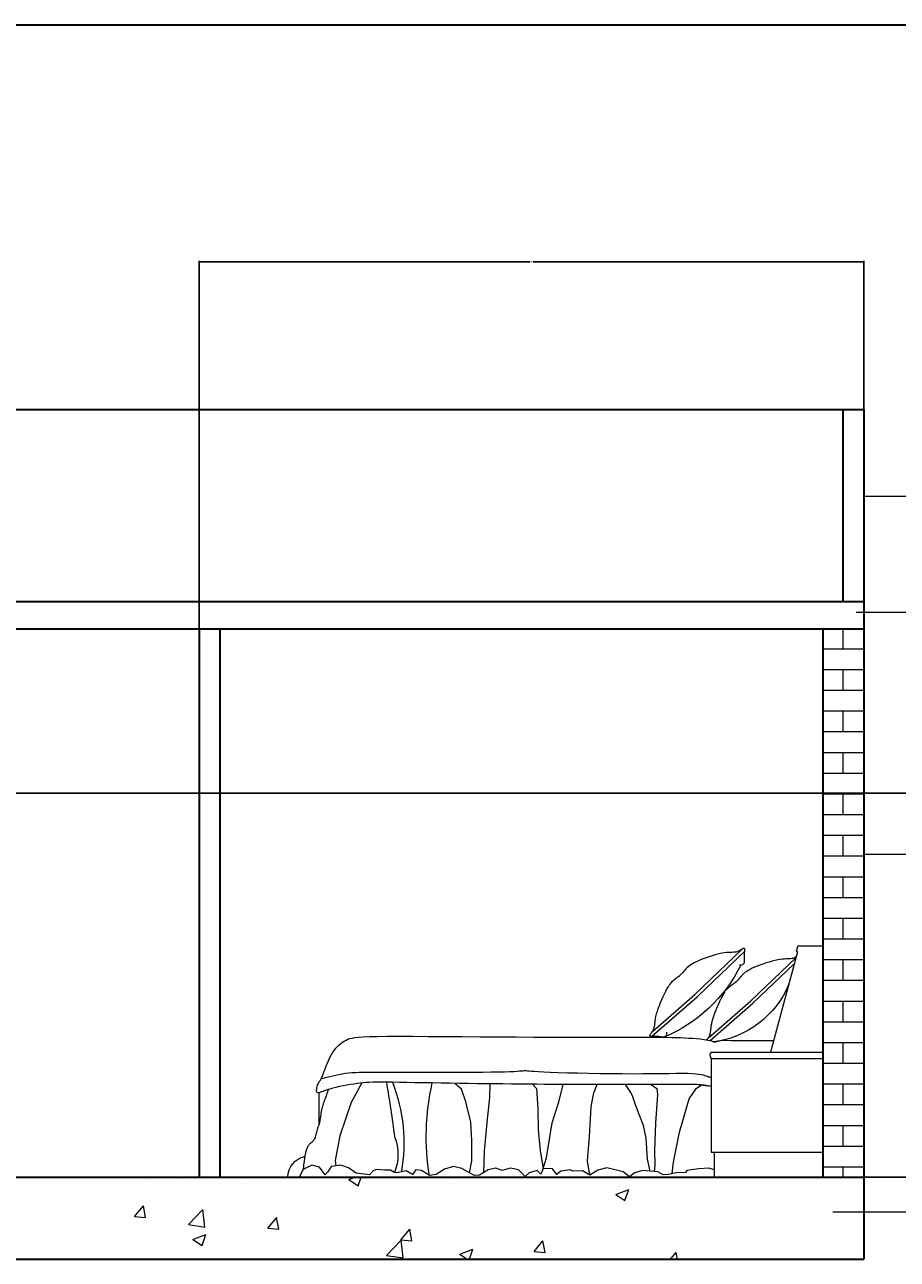
# Model space of a CAD drawing. Units: inches. Extents: x 2250 to 3547, y 1387 to 2604.
# Tile 10 of 11: x 3100 to 3291, y 2334 to 2604. Entities that reach past the tile are written whole.
import ezdxf

# ---------------------------------------------------------------- set-up
doc = ezdxf.new("R2010")
doc.units = ezdxf.units.IN
for name, color, linetype, lineweight in [('A-ANNO-DIMS', 2, 'Continuous', 18), ('A-ANNO-TEXT', 7, 'Continuous', 18), ('A-ANNO-TTLB', 7, 'Continuous', 35), ('A-FLOR-PATT', 252, 'Continuous', 13), ('A-FURN', 9, 'Continuous', 18), ('A-SECT', 7, 'Continuous', 35), ('A-WALL-PATT', 252, 'Continuous', 13)]:
    doc.layers.add(name, color=color, linetype=linetype, lineweight=lineweight)
doc.styles.get("Standard").update_dxf_attribs({"font": 'arial.ttf'})
doc.dimstyles.get("Standard").update_dxf_attribs({"dimtxt": 0.18, "dimasz": 0.18, "dimexe": 0.18, "dimexo": 0.0625, "dimgap": 0.09, "dimtad": 0, "dimtih": 1, "dimtoh": 1, "dimdec": 4, "dimzin": 0, "dimdsep": 46, "dimtxsty": 'Standard', "dimcen": 0.09, "dimadec": 0, "dimazin": 0, "dimtfac": 1, "dimtdec": 4, "dimtofl": 0, "dimtmove": 0, "dimatfit": 3, "dimfxl": 1, "dimtolj": 1, "dimtzin": 0, "dimarcsym": 0})

# ---------------------------------------------------------------- blocks, each defined once
blk = doc.blocks.new('A$C08BC4B9A')
for p, q in [((0, 924.5), (0.5, 925)), ((0, 0), (0, 924.5)), ((95, 925), (0.5, 925)), ((101.1, 921.9), (105, 907.4)), ((101.4, 901.2), (208.9, 500)), ((311.4, 909.3), (311.5, 910.8)), ((311.5, 907.6), (311.4, 909.3)), ((311.5, 910.8), (311.7, 912.1)), ((311.7, 905.6), (311.5, 907.6)), ((311.7, 912.1), (312.1, 913.2)), ((312, 903.5), (311.7, 905.6)), ((502.9, 721.7), (311.9, 904.5)), ((312.3, 901.1), (312, 903.5)), ((312.1, 913.2), (312.7, 914.1)), ((312.6, 898.6), (312.3, 901.1)), ((312.9, 895.9), (312.6, 898.6)), ((312.7, 914.1), (313.6, 914.7)), ((313.1, 892.9), (312.9, 895.9)), ((313.3, 889.8), (313.1, 892.9)), ((313.4, 886.5), (313.3, 889.8)), ((313.6, 914.7), (314.7, 915)), ((314.7, 915), (316, 915.1)), ((316, 915.1), (317.6, 914.9)), ((317.6, 914.9), (319.3, 914.5)), ((319.3, 914.5), (321.1, 913.7)), ((511.6, 731.1), (320.5, 913.9)), ((321.1, 913.7), (323.2, 912.6)), ((323.2, 912.6), (325.4, 911.2)), ((325.4, 911.2), (327.8, 909.6)), ((327.8, 909.6), (330.4, 907.8)), ((330.4, 907.8), (333.3, 906.1)), ((333.3, 906.1), (336.4, 904.3)), ((336.4, 904.3), (339.9, 902.7)), ((339.9, 902.7), (343.7, 901.4)), ((343.7, 901.4), (347.9, 900.4)), ((347.9, 900.4), (352.5, 899.8)), ((352.5, 899.8), (357.6, 899.5)), ((357.6, 899.5), (363.2, 899.4)), ((363.2, 899.4), (369.6, 899.2)), ((369.6, 899.2), (376.7, 898.9)), ((376.7, 898.9), (384.6, 898.3)), ((384.6, 898.3), (393.4, 897.3)), ((393.4, 897.3), (403.3, 895.7)), ((403.3, 895.7), (414.2, 893.3)), ((414.2, 893.3), (425.9, 890.4)), ((425.9, 890.4), (438.1, 886.9)), ((106.6, 881.7), (106.8, 881.6)), ((106.8, 881.6), (109.7, 879.8)), ((288, 704.9), (107.8, 877.3)), ((109.7, 879.8), (112.8, 878.1)), ((112.8, 878.1), (116.3, 876.5)), ((279.2, 695.5), (114.2, 853.4)), ((116.3, 876.5), (120.1, 875.2)), ((120.1, 875.2), (124.3, 874.2)), ((124.3, 874.2), (128.9, 873.6)), ((128.9, 873.6), (134, 873.3)), ((134, 873.3), (139.6, 873.2)), ((139.6, 873.2), (146, 873)), ((146, 873), (153.1, 872.7)), ((153.1, 872.7), (161, 872.1)), ((161, 872.1), (169.8, 871.1)), ((169.8, 871.1), (179.7, 869.5)), ((179.7, 869.5), (190.6, 867.1)), ((190.6, 867.1), (202.3, 864.2)), ((202.3, 864.2), (214.5, 860.7)), ((214.5, 860.7), (226.9, 856.8)), ((226.9, 856.8), (239.3, 852.7)), ((239.3, 852.7), (251.3, 848.4)), ((251.3, 848.4), (262.7, 844)), ((262.7, 844), (273.2, 839.6)), ((312.7, 863.2), (312.8, 867.3)), ((313.1, 859.2), (312.7, 863.2)), ((312.8, 867.3), (313, 871.5)), ((313, 871.5), (313.3, 875.5)), ((314.3, 855.7), (313.1, 859.2)), ((313.3, 875.5), (313.4, 879.4)), ((313.4, 883), (313.4, 886.5)), ((313.4, 879.4), (313.4, 883)), ((316.7, 852.8), (314.3, 855.7)), ((320.4, 850.8), (316.7, 852.8)), ((325.8, 849.7), (320.4, 850.8)), ((333.2, 849.9), (325.8, 849.7)), ((438.1, 886.9), (450.5, 883.1)), ((450.5, 883.1), (462.9, 878.9)), ((462.9, 878.9), (474.9, 874.6)), ((474.9, 874.6), (486.3, 870.2)), ((486.3, 870.2), (496.8, 865.9)), ((496.8, 865.9), (506.1, 861.7)), ((506.1, 861.7), (514.3, 857.6)), ((514.3, 857.6), (521.6, 853.6)), ((521.6, 853.6), (528, 849.7)), ((528, 849.7), (533.7, 845.7)), ((533.7, 845.7), (538.8, 841.7)), ((538.8, 841.7), (543.4, 837.5)), ((273.2, 839.6), (282.5, 835.5)), ((282.5, 835.5), (290.7, 831.4)), ((290.7, 831.4), (298, 827.4)), ((298, 827.4), (304.4, 823.4)), ((304.4, 823.4), (310.1, 819.5)), ((310.1, 819.5), (315.2, 815.4)), ((315.2, 815.4), (319.8, 811.3)), ((319.8, 811.3), (324.1, 807)), ((324.1, 807), (328.1, 802.5)), ((328.1, 802.5), (332, 797.9)), ((332, 797.9), (335.8, 793.2)), ((335.8, 793.2), (339.7, 788.4)), ((543.4, 837.5), (547.7, 833.2)), ((547.7, 833.2), (551.7, 828.7)), ((551.7, 828.7), (555.6, 824.1)), ((555.6, 824.1), (559.4, 819.4)), ((559.4, 819.4), (563.3, 814.6)), ((563.3, 814.6), (567.7, 810.4)), ((572.2, 806.3), (567.7, 810.4)), ((577.3, 802.8), (572.2, 806.3)), ((582.3, 799.4), (577.3, 802.8)), ((587.2, 795.8), (582.3, 799.4)), ((592, 792.2), (587.2, 795.8)), ((596.6, 788.2), (592, 792.2)), ((339.7, 788.4), (344.1, 784.1)), ((344.2, 784), (344.1, 784.1)), ((344.5, 783.8), (344.2, 784)), ((344.9, 783.4), (344.5, 783.8)), ((345.5, 782.9), (344.9, 783.4)), ((346.1, 782.3), (345.5, 782.9)), ((346.8, 781.7), (346.1, 782.3)), ((347.6, 781.1), (346.8, 781.7)), ((348.3, 780.5), (347.6, 781.1)), ((349.1, 779.9), (348.3, 780.5)), ((349.8, 779.4), (349.1, 779.9)), ((350.5, 778.9), (349.8, 779.4)), ((351.1, 778.4), (350.5, 778.9)), ((351.8, 777.9), (351.1, 778.4)), ((352.4, 777.5), (351.8, 777.9)), ((353.1, 777), (352.4, 777.5)), ((353.7, 776.6), (353.1, 777)), ((354.3, 776.2), (353.7, 776.6)), ((354.9, 775.7), (354.3, 776.2)), ((355.6, 775.3), (354.9, 775.7)), ((356.2, 774.9), (355.6, 775.3)), ((356.8, 774.4), (356.2, 774.9)), ((357.4, 774), (356.8, 774.4)), ((358.1, 773.6), (357.4, 774)), ((358.7, 773.1), (358.1, 773.6)), ((359.3, 772.7), (358.7, 773.1)), ((359.9, 772.3), (359.3, 772.7)), ((360.5, 771.8), (359.9, 772.3)), ((361.2, 771.4), (360.5, 771.8)), ((361.8, 770.9), (361.2, 771.4)), ((362.4, 770.5), (361.8, 770.9)), ((363, 770), (362.4, 770.5)), ((363.6, 769.6), (363, 770)), ((364.2, 769.1), (363.6, 769.6)), ((364.8, 768.7), (364.2, 769.1)), ((365.4, 768.2), (364.8, 768.7)), ((366, 767.8), (365.4, 768.2)), ((366.6, 767.3), (366, 767.8)), ((367.2, 766.8), (366.6, 767.3)), ((367.8, 766.4), (367.2, 766.8)), ((368.3, 765.9), (367.8, 766.4)), ((368.9, 765.4), (368.3, 765.9)), ((369.5, 764.9), (368.9, 765.4)), ((370.1, 764.4), (369.5, 764.9)), ((370.7, 763.9), (370.1, 764.4)), ((371.2, 763.5), (370.7, 763.9)), ((371.8, 763), (371.2, 763.5)), ((372.4, 762.4), (371.8, 763)), ((373, 761.9), (372.4, 762.4)), ((373.5, 761.4), (373, 761.9)), ((374.1, 760.9), (373.5, 761.4)), ((374.7, 760.4), (374.1, 760.9)), ((375.2, 759.8), (374.7, 760.4)), ((375.8, 759.3), (375.2, 759.8)), ((376.3, 758.7), (375.8, 759.3)), ((376.9, 758.2), (376.3, 758.7)), ((377.4, 757.6), (376.9, 758.2)), ((378, 757), (377.4, 757.6)), ((378.6, 756.5), (378, 757)), ((379.2, 755.8), (378.6, 756.5)), ((379.8, 755.2), (379.2, 755.8)), ((380.5, 754.5), (379.8, 755.2)), ((381.3, 753.8), (380.5, 754.5)), ((382.2, 753.1), (381.3, 753.8)), ((383.2, 752.3), (382.2, 753.1)), ((384.2, 751.4), (383.2, 752.3)), ((385.4, 750.5), (384.2, 751.4)), ((386.6, 749.6), (385.4, 750.5)), ((387.8, 748.7), (386.6, 749.6)), ((388.9, 747.8), (387.8, 748.7)), ((389.9, 746.9), (388.9, 747.8)), ((390.8, 746), (389.9, 746.9)), ((391.4, 745.3), (390.8, 746)), ((391.9, 744.6), (391.4, 745.3)), ((392.1, 744), (391.9, 744.6)), ((392, 741.9), (392.1, 742.4)), ((392, 741.3), (392, 741.9)), ((392, 740.8), (392, 741.3)), ((392.2, 743.4), (392.1, 744)), ((392.1, 742.4), (392.2, 742.9)), ((392.2, 742.9), (392.2, 743.4)), ((601.1, 783.9), (596.6, 788.2)), ((605.5, 779.1), (601.1, 783.9)), ((609.9, 773.7), (605.5, 779.1)), ((614.3, 767.6), (609.9, 773.7)), ((618.8, 760.7), (614.3, 767.6)), ((623.5, 752.8), (618.8, 760.7)), ((628.4, 743.8), (623.5, 752.8)), ((633.5, 733.7), (628.4, 743.8)), ((450.1, 546.6), (279.2, 695.5)), ((457.7, 557), (288, 704.9)), ((392.1, 740.1), (392, 740.8)), ((392.4, 739.4), (392.1, 740.1)), ((392.7, 738.6), (392.4, 739.4)), ((393.1, 737.8), (392.7, 738.6)), ((393.6, 737), (393.1, 737.8)), ((394.1, 736.1), (393.6, 737)), ((394.7, 735.2), (394.1, 736.1)), ((395.2, 734.3), (394.7, 735.2)), ((395.8, 733.4), (395.2, 734.3)), ((396.4, 732.4), (395.8, 733.4)), ((397, 731.5), (396.4, 732.4)), ((397.6, 730.5), (397, 731.5)), ((398.2, 729.5), (397.6, 730.5)), ((398.7, 728.5), (398.2, 729.5)), ((399.3, 727.4), (398.7, 728.5)), ((399.9, 726.4), (399.3, 727.4)), ((400.5, 725.3), (399.9, 726.4)), ((401.1, 724.3), (400.5, 725.3)), ((401.7, 723.2), (401.1, 724.3)), ((402.4, 722), (401.7, 723.2)), ((403, 720.9), (402.4, 722)), ((403.6, 719.8), (403, 720.9)), ((404.2, 718.6), (403.6, 719.8)), ((404.8, 717.4), (404.2, 718.6)), ((405.4, 716.2), (404.8, 717.4)), ((406.1, 715), (405.4, 716.2)), ((406.7, 713.8), (406.1, 715)), ((407.3, 712.5), (406.7, 713.8)), ((408, 711.2), (407.3, 712.5)), ((408.6, 710), (408, 711.2)), ((409.3, 708.7), (408.6, 710)), ((409.9, 707.3), (409.3, 708.7)), ((410.6, 706), (409.9, 707.3)), ((411.2, 704.7), (410.6, 706)), ((411.9, 703.3), (411.2, 704.7)), ((412.5, 701.9), (411.9, 703.3)), ((413.2, 700.6), (412.5, 701.9)), ((413.8, 699.2), (413.2, 700.6)), ((414.5, 697.8), (413.8, 699.2)), ((415.1, 696.4), (414.5, 697.8)), ((415.8, 694.9), (415.1, 696.4)), ((416.4, 693.5), (415.8, 694.9)), ((417.1, 692.1), (416.4, 693.5)), ((417.7, 690.6), (417.1, 692.1)), ((685.7, 562.3), (502.9, 721.7)), ((681.3, 583.2), (511.6, 731.1)), ((638.7, 722.7), (633.5, 733.7)), ((643.9, 711), (638.7, 722.7)), ((649, 699), (643.9, 711)), ((653.8, 686.9), (649, 699)), ((418.4, 689.2), (417.7, 690.6)), ((419, 687.7), (418.4, 689.2)), ((419.7, 686.2), (419, 687.7)), ((420.3, 684.7), (419.7, 686.2)), ((421, 683.3), (420.3, 684.7)), ((421.6, 681.8), (421, 683.3)), ((422.2, 680.3), (421.6, 681.8)), ((422.9, 678.8), (422.2, 680.3)), ((423.5, 677.3), (422.9, 678.8)), ((424.1, 675.8), (423.5, 677.3)), ((424.7, 674.3), (424.1, 675.8)), ((425.4, 672.8), (424.7, 674.3)), ((426, 671.3), (425.4, 672.8)), ((426.6, 669.7), (426, 671.3)), ((427.2, 668.2), (426.6, 669.7)), ((427.8, 666.7), (427.2, 668.2)), ((428.4, 665.2), (427.8, 666.7)), ((429, 663.7), (428.4, 665.2)), ((429.6, 662.2), (429, 663.7)), ((430.1, 660.7), (429.6, 662.2)), ((430.7, 659.2), (430.1, 660.7)), ((431.3, 657.7), (430.7, 659.2)), ((431.8, 656.2), (431.3, 657.7)), ((432.4, 654.7), (431.8, 656.2)), ((432.9, 653.2), (432.4, 654.7)), ((433.4, 651.8), (432.9, 653.2)), ((434, 650.3), (433.4, 651.8)), ((434.5, 648.8), (434, 650.3)), ((435, 647.4), (434.5, 648.8)), ((435.5, 645.9), (435, 647.4)), ((436, 644.5), (435.5, 645.9)), ((436.5, 643.1), (436, 644.5)), ((436.9, 641.7), (436.5, 643.1)), ((658.2, 675), (653.8, 686.9)), ((662, 663.6), (658.2, 675)), ((665.2, 652.9), (662, 663.6)), ((667.5, 643.2), (665.2, 652.9)), ((669.2, 634.4), (667.5, 643.2)), ((437.4, 640.2), (436.9, 641.7)), ((437.9, 638.8), (437.4, 640.2)), ((438.3, 637.5), (437.9, 638.8)), ((438.7, 636.1), (438.3, 637.5)), ((439.1, 634.7), (438.7, 636.1)), ((439.6, 633.4), (439.1, 634.7)), ((440, 632), (439.6, 633.4)), ((440.3, 630.7), (440, 632)), ((440.7, 629.4), (440.3, 630.7)), ((441.1, 628.1), (440.7, 629.4)), ((441.4, 626.8), (441.1, 628.1)), ((441.8, 625.5), (441.4, 626.8)), ((442.1, 624.3), (441.8, 625.5)), ((442.4, 623.1), (442.1, 624.3)), ((442.7, 621.8), (442.4, 623.1)), ((443, 620.6), (442.7, 621.8)), ((443.3, 619.4), (443, 620.6)), ((443.6, 618.3), (443.3, 619.4)), ((443.8, 617.1), (443.6, 618.3)), ((444.1, 616), (443.8, 617.1)), ((444.3, 614.8), (444.1, 616)), ((444.5, 613.7), (444.3, 614.8)), ((444.7, 612.6), (444.5, 613.7)), ((445, 611.5), (444.7, 612.6)), ((445.2, 610.5), (445, 611.5)), ((445.4, 609.4), (445.2, 610.5)), ((445.5, 608.4), (445.4, 609.4)), ((445.7, 607.3), (445.5, 608.4)), ((445.9, 606.3), (445.7, 607.3)), ((446, 605.3), (445.9, 606.3)), ((446.2, 604.3), (446, 605.3)), ((446.4, 603.3), (446.2, 604.3)), ((446.5, 602.4), (446.4, 603.3)), ((446.6, 601.4), (446.5, 602.4)), ((446.8, 600.5), (446.6, 601.4)), ((446.9, 599.6), (446.8, 600.5)), ((447, 598.6), (446.9, 599.6)), ((447.1, 597.7), (447, 598.6)), ((447.2, 596.9), (447.1, 597.7)), ((447.3, 596), (447.2, 596.9)), ((447.4, 595.1), (447.3, 596)), ((447.5, 594.3), (447.4, 595.1)), ((447.6, 593.4), (447.5, 594.3)), ((447.7, 592.6), (447.6, 593.4)), ((670.4, 626.6), (669.2, 634.4)), ((671.3, 619.5), (670.4, 626.6)), ((671.9, 613.2), (671.3, 619.5)), ((672.5, 607.6), (671.9, 613.2)), ((673.1, 602.5), (672.5, 607.6)), ((674.1, 598), (673.1, 602.5)), ((675.4, 593.9), (674.1, 598)), ((677, 590.2), (675.4, 593.9)), ((366.1, 546.8), (196.6, 546.1)), ((400.7, 547.5), (366.1, 546.8)), ((420, 543.6), (400.7, 547.5)), ((431.7, 540.1), (420, 543.6)), ((445.4, 545.7), (439.4, 542.5)), ((460.2, 548.4), (445.4, 545.7)), ((447.8, 591.8), (447.7, 592.6)), ((447.9, 591), (447.8, 591.8)), ((448, 590.2), (447.9, 591)), ((448, 589.4), (448, 590.2)), ((448.1, 588.6), (448, 589.4)), ((448.2, 587.9), (448.1, 588.6)), ((448.3, 587.1), (448.2, 587.9)), ((448.3, 586.4), (448.3, 587.1)), ((448.4, 585.6), (448.3, 586.4)), ((448.5, 584.9), (448.4, 585.6)), ((448.6, 584.2), (448.5, 584.9)), ((448.6, 583.5), (448.6, 584.2)), ((448.7, 582.8), (448.6, 583.5)), ((448.8, 582.1), (448.7, 582.8)), ((448.9, 581.4), (448.8, 582.1)), ((448.9, 580.8), (448.9, 581.4)), ((449, 580.1), (448.9, 580.8)), ((449.1, 579.5), (449, 580.1)), ((449.2, 578.8), (449.1, 579.5)), ((449.3, 578.2), (449.2, 578.8)), ((449.4, 577.6), (449.3, 578.2)), ((449.5, 577), (449.4, 577.6)), ((449.6, 576.4), (449.5, 577)), ((449.7, 575.8), (449.6, 576.4)), ((449.8, 575.2), (449.7, 575.8)), ((449.9, 574.6), (449.8, 575.2)), ((450, 574), (449.9, 574.6)), ((450.1, 573.5), (450, 574)), ((450.3, 572.9), (450.1, 573.5)), ((450.4, 572.4), (450.3, 572.9)), ((450.5, 571.8), (450.4, 572.4)), ((450.7, 571.3), (450.5, 571.8)), ((450.8, 570.8), (450.7, 571.3)), ((451, 570.2), (450.8, 570.8)), ((451.1, 569.7), (451, 570.2)), ((451.3, 569.2), (451.1, 569.7)), ((451.5, 568.7), (451.3, 569.2)), ((451.6, 568.2), (451.5, 568.7)), ((451.8, 567.7), (451.6, 568.2)), ((452, 567.2), (451.8, 567.7)), ((452.2, 566.8), (452, 567.2)), ((452.4, 566.3), (452.2, 566.8)), ((452.6, 565.8), (452.4, 566.3)), ((452.8, 565.4), (452.6, 565.8)), ((453, 564.9), (452.8, 565.4)), ((453.2, 564.5), (453, 564.9)), ((453.4, 564), (453.2, 564.5)), ((453.6, 563.6), (453.4, 564)), ((453.8, 563.1), (453.6, 563.6)), ((454.1, 562.7), (453.8, 563.1)), ((454.3, 562.3), (454.1, 562.7)), ((454.5, 561.9), (454.3, 562.3)), ((454.8, 561.5), (454.5, 561.9)), ((455, 561.1), (454.8, 561.5)), ((455.2, 560.7), (455, 561.1)), ((455.5, 560.3), (455.2, 560.7)), ((455.7, 559.9), (455.5, 560.3)), ((456, 559.5), (455.7, 559.9)), ((456.2, 559.1), (456, 559.5)), ((456.4, 558.8), (456.2, 559.1)), ((456.7, 558.4), (456.4, 558.8)), ((456.9, 558), (456.7, 558.4)), ((457.2, 557.7), (456.9, 558)), ((457.4, 557.3), (457.2, 557.7)), ((457.7, 557), (457.4, 557.3)), ((457.9, 556.6), (457.7, 557)), ((458.2, 556.3), (457.9, 556.6)), ((458.4, 555.9), (458.2, 556.3)), ((458.7, 555.6), (458.4, 555.9)), ((458.9, 555.3), (458.7, 555.6)), ((459.2, 554.9), (458.9, 555.3)), ((459.4, 554.6), (459.2, 554.9)), ((459.7, 554.3), (459.4, 554.6)), ((459.9, 554), (459.7, 554.3)), ((460.2, 553.6), (459.9, 554)), ((460.4, 553.3), (460.2, 553.6)), ((475.2, 550.7), (460.2, 548.4)), ((460.7, 553), (460.4, 553.3)), ((461, 552.6), (460.7, 553)), ((461.3, 552.3), (461, 552.6)), ((461.6, 551.9), (461.3, 552.3)), ((461.9, 551.5), (461.6, 551.9)), ((462.2, 551.1), (461.9, 551.5)), ((462.5, 550.7), (462.2, 551.1)), ((462.8, 550.3), (462.5, 550.7)), ((463.2, 549.8), (462.8, 550.3)), ((463.5, 549.4), (463.2, 549.8)), ((463.8, 548.9), (463.5, 549.4)), ((490.5, 552.6), (475.2, 550.7)), ((506, 554.2), (490.5, 552.6)), ((521.7, 555.5), (506, 554.2)), ((537.6, 556.6), (521.7, 555.5)), ((553.6, 557.4), (537.6, 556.6)), ((569.7, 558.1), (553.6, 557.4)), ((586, 558.6), (569.7, 558.1)), ((603.2, 559), (586, 558.6)), ((621.8, 559.3), (603.2, 559)), ((642.6, 559.5), (621.8, 559.3)), ((624.8, 579.5), (625.2, 572.1)), ((625.2, 572.1), (626.6, 566.8)), ((626.6, 566.8), (629, 563.3)), ((629, 563.3), (632, 561.2)), ((632, 561.2), (635.6, 560.2)), ((635.6, 560.2), (639.6, 560.1)), ((639.6, 560.1), (643.7, 560.5)), ((666.5, 559.6), (642.6, 559.5)), ((643.7, 560.5), (647.9, 561)), ((647.9, 561), (651.9, 561.6)), ((651.9, 561.6), (655.7, 562)), ((655.7, 562), (659.3, 562.3)), ((659.3, 562.3), (662.8, 562.5)), ((662.8, 562.5), (666.1, 562.7)), ((666.1, 562.7), (669.2, 562.7)), ((693.9, 559.6), (666.5, 559.6)), ((669.2, 562.7), (672.2, 562.7)), ((672.2, 562.7), (674.9, 562.7)), ((674.9, 562.7), (677.5, 562.6)), ((678.8, 586.8), (677, 590.2)), ((677.5, 562.6), (679.8, 562.4)), ((680.8, 583.8), (678.8, 586.8)), ((679.8, 562.4), (682, 562.3)), ((682.8, 581.1), (680.8, 583.8)), ((682, 562.3), (683.9, 562.3)), ((684.7, 578.6), (682.8, 581.1)), ((683.9, 562.3), (685.7, 562.3)), ((686.5, 576.4), (684.7, 578.6)), ((685.7, 562.3), (687.2, 562.4)), ((688.1, 574.3), (686.5, 576.4)), ((687.2, 562.4), (688.5, 562.7)), ((689.3, 572.3), (688.1, 574.3)), ((688.5, 562.7), (689.5, 563.2)), ((690.2, 570.5), (689.3, 572.3)), ((689.5, 563.2), (690.3, 563.9)), ((690.8, 568.8), (690.2, 570.5)), ((690.3, 563.9), (690.9, 564.9)), ((691.1, 567.3), (690.8, 568.8)), ((690.9, 564.9), (691.1, 566)), ((691.1, 566), (691.1, 567.3)), ((725.8, 559.7), (693.9, 559.6)), ((762.8, 559.7), (725.8, 559.7)), ((805.4, 559.7), (762.8, 559.7)), ((853.4, 559.7), (805.4, 559.7)), ((906.2, 559.7), (853.4, 559.7)), ((963.4, 559.8), (906.2, 559.7)), ((1024.6, 559.9), (963.4, 559.8)), ((1089.2, 560.1), (1024.6, 559.9)), ((1156.7, 560.4), (1089.2, 560.1)), ((1226.8, 560.7), (1156.7, 560.4)), ((1298.7, 561.1), (1226.8, 560.7)), ((1371.2, 561.6), (1298.7, 561.1)), ((1443.1, 562.1), (1371.2, 561.6)), ((1512.8, 562.6), (1443.1, 562.1)), ((1579.1, 563), (1512.8, 562.6)), ((1640.5, 563.3), (1579.1, 563)), ((1695.8, 563.4), (1640.5, 563.3)), ((1743.5, 563.3), (1695.8, 563.4)), ((1782.8, 563), (1743.5, 563.3)), ((1814.2, 562.4), (1782.8, 563)), ((1838.9, 561.5), (1814.2, 562.4)), ((1858, 560.2), (1838.9, 561.5)), ((1872.6, 558.6), (1858, 560.2)), ((1883.7, 556.6), (1872.6, 558.6)), ((1892.6, 554.2), (1883.7, 556.6)), ((1900.3, 551.3), (1892.6, 554.2)), ((1907.7, 547.9), (1900.3, 551.3)), ((1915, 544), (1907.7, 547.9)), ((1922.1, 539.6), (1915, 544)), ((445.9, 500), (0, 500)), ((439.4, 542.5), (431.7, 540.1)), ((1929, 534.5), (1922.1, 539.6)), ((1935.8, 528.9), (1929, 534.5)), ((1942.3, 522.6), (1935.8, 528.9)), ((1948.6, 515.6), (1942.3, 522.6)), ((1954.6, 508), (1948.6, 515.6)), ((1960.4, 499.6), (1954.6, 508)), ((1965.8, 490.7), (1960.4, 499.6)), ((445.9, 475), (0, 475)), ((445.9, 475), (445.9, 100)), ((1970.9, 481.5), (1965.8, 490.7)), ((1975.6, 472.1), (1970.9, 481.5)), ((1980, 462.7), (1975.6, 472.1)), ((1984, 453.6), (1980, 462.7)), ((1987.5, 445), (1984, 453.6)), ((1990.7, 437), (1987.5, 445)), ((445.9, 397.8), (449.1, 398.3)), ((449.1, 398.3), (453.4, 399.2)), ((453.4, 399.2), (457.6, 400.4)), ((457.6, 400.4), (461.8, 402)), ((461.8, 402), (466.2, 403.7)), ((466.2, 403.7), (471.3, 405.6)), ((471.3, 405.6), (477.6, 407.5)), ((477.6, 407.5), (485.4, 409.4)), ((485.4, 409.4), (495.3, 411.1)), ((495.3, 411.1), (507.7, 412.5)), ((507.7, 412.5), (523, 413.5)), ((523, 413.5), (541.5, 414)), ((541.5, 414), (563.2, 414.2)), ((563.2, 414.2), (588.2, 414.1)), ((588.2, 414.1), (616.4, 413.7)), ((616.4, 413.7), (647.7, 413.3)), ((647.7, 413.3), (682, 412.9)), ((682, 412.9), (719.4, 412.6)), ((719.4, 412.6), (759.7, 412.4)), ((759.7, 412.4), (802.6, 412.6)), ((802.6, 412.6), (847.4, 413)), ((847.4, 413), (892.8, 413.6)), ((892.8, 413.6), (937.8, 414.4)), ((937.8, 414.4), (981.1, 415.3)), ((981.1, 415.3), (1021.7, 416.4)), ((1021.7, 416.4), (1058.6, 417.5)), ((1058.6, 417.5), (1090.4, 418.7)), ((1090.4, 418.7), (1116.5, 419.9)), ((1116.5, 419.9), (1137.2, 421)), ((1137.2, 421), (1153.4, 422.1)), ((1153.4, 422.1), (1165.7, 423)), ((1165.7, 423), (1174.9, 423.8)), ((1174.9, 423.8), (1181.7, 424.4)), ((1181.7, 424.4), (1186.9, 424.8)), ((1186.9, 424.8), (1191.2, 425)), ((1191.2, 425), (1195.4, 424.8)), ((1195.4, 424.8), (1200, 424.5)), ((1200, 424.5), (1205.8, 423.9)), ((1205.8, 423.9), (1213.3, 423.2)), ((1213.3, 423.2), (1223.1, 422.4)), ((1223.1, 422.4), (1236, 421.7)), ((1236, 421.7), (1252.5, 420.9)), ((1252.5, 420.9), (1273.3, 420.3)), ((1273.3, 420.3), (1298.7, 419.7)), ((1298.7, 419.7), (1328.3, 419.4)), ((1328.3, 419.4), (1361.1, 419.1)), ((1361.1, 419.1), (1396.4, 418.9)), ((1396.4, 418.9), (1433.4, 418.8)), ((1433.4, 418.8), (1471.3, 418.7)), ((1471.3, 418.7), (1509.3, 418.7)), ((1509.3, 418.7), (1546.6, 418.7)), ((1546.6, 418.7), (1582.4, 418.7)), ((1582.4, 418.7), (1616.7, 418.7)), ((1616.7, 418.7), (1649.3, 418.7)), ((1649.3, 418.7), (1680.1, 418.7)), ((1680.1, 418.7), (1709, 418.7)), ((1709, 418.7), (1736, 418.7)), ((1736, 418.7), (1760.9, 418.7)), ((1760.9, 418.7), (1783.8, 418.7)), ((1783.8, 418.7), (1804.5, 418.7)), ((1804.5, 418.7), (1823.2, 418.6)), ((1823.2, 418.6), (1840.3, 418.5)), ((1840.3, 418.5), (1856.1, 418.1)), ((1856.1, 418.1), (1870.7, 417.6)), ((1870.7, 417.6), (1884.5, 416.7)), ((1884.5, 416.7), (1897.8, 415.6)), ((1897.8, 415.6), (1910.8, 414)), ((1910.8, 414), (1923.7, 412)), ((1923.7, 412), (1936.5, 409.7)), ((1936.5, 409.7), (1949.1, 407.1)), ((1949.1, 407.1), (1961.3, 404.4)), ((1961.3, 404.4), (1973.1, 401.6)), ((1973.1, 401.6), (1984.4, 398.8)), ((1984.4, 398.8), (1995, 396.1)), ((1993.4, 429.7), (1990.7, 437)), ((1995.8, 423.3), (1993.4, 429.7)), ((1995, 396.1), (2004.8, 393.6)), ((1997.8, 417.5), (1995.8, 423.3)), ((1999.6, 412.4), (1997.8, 417.5)), ((2001.3, 407.8), (1999.6, 412.4)), ((2002.8, 403.7), (2001.3, 407.8)), ((2004.3, 400.1), (2002.8, 403.7)), ((2005.8, 396.8), (2004.3, 400.1)), ((2007.5, 393.8), (2005.8, 396.8)), ((445.9, 362), (481.5, 369.7)), ((445.9, 362.5), (450.4, 363.2)), ((450.4, 363.2), (457.2, 364.1)), ((457.2, 364.1), (463.4, 364.9)), ((463.4, 364.9), (468.9, 365.7)), ((468.9, 365.7), (473.6, 366.4)), ((473.6, 366.4), (477.6, 367.1)), ((477.6, 367.1), (481.1, 367.7)), ((481.1, 367.7), (484.4, 368.3)), ((484.4, 368.3), (488, 368.8)), ((504.7, 356.4), (486.2, 368.5)), ((488, 368.8), (492.3, 369.2)), ((492.3, 369.2), (497.5, 369.6)), ((497.5, 369.6), (504.1, 369.9)), ((504.1, 369.9), (512.5, 370.1)), ((534.3, 312.8), (504.7, 356.4)), ((512.5, 370.1), (522.9, 370.3)), ((522.9, 370.3), (535.3, 370.3)), ((535.3, 370.3), (549.5, 370.3)), ((549.5, 370.3), (565.4, 370.3)), ((565.4, 370.3), (582.8, 370.2)), ((582.8, 370.2), (601.6, 370.2)), ((601.6, 370.2), (621.6, 370.1)), ((621.6, 370.1), (642.7, 370.1)), ((642.7, 370.1), (664.7, 370.1)), ((663.6, 354.7), (661.8, 330.2)), ((687.3, 370.2), (663.6, 354.7)), ((664.7, 370.1), (687.3, 370.2)), ((687.3, 370.2), (710.4, 370.3)), ((710.4, 370.3), (733.4, 370.4)), ((733.4, 370.4), (756.3, 370.4)), ((756.3, 370.4), (778.7, 370.5)), ((768.3, 339), (789.4, 370.5)), ((778.7, 370.5), (800.2, 370.6)), ((800.2, 370.6), (820.7, 370.6)), ((820.7, 370.6), (840, 370.6)), ((840, 370.6), (858.3, 370.5)), ((858.3, 370.5), (876.2, 370.4)), ((876.2, 370.4), (894, 370.4)), ((894, 370.4), (912.3, 370.3)), ((916.7, 337.2), (903.2, 370.3)), ((912.3, 370.3), (931.5, 370.2)), ((931.5, 370.2), (952, 370.2)), ((952, 370.2), (974.3, 370.2)), ((974.3, 370.2), (998.7, 370.3)), ((998.7, 370.3), (1025.1, 370.4)), ((1025.1, 370.4), (1053.2, 370.6)), ((1054.7, 305.8), (1039.1, 370.5)), ((1053.2, 370.6), (1082.9, 370.8)), ((1082.9, 370.8), (1113.8, 371)), ((1113.8, 371), (1145.8, 371.3)), ((1145.5, 354.7), (1140.2, 274.4)), ((1162.2, 371.4), (1145.5, 354.7)), ((1145.8, 371.3), (1178.6, 371.6)), ((1178.6, 371.6), (1212, 371.9)), ((1212, 371.9), (1245.7, 372.2)), ((1245.7, 372.2), (1279.8, 372.6)), ((1279.8, 372.6), (1314.1, 373)), ((1314.1, 373), (1348.8, 373.4)), ((1332.3, 318), (1331.5, 373.2)), ((1348.8, 373.4), (1383.8, 373.8)), ((1383.8, 373.8), (1419.1, 374.3)), ((1419.1, 374.3), (1454.7, 374.8)), ((1428.3, 300.6), (1445.8, 351.2)), ((1445.8, 351.2), (1472.7, 375.1)), ((1454.7, 374.8), (1490.6, 375.4)), ((1490.6, 375.4), (1526.8, 376)), ((1526.8, 376), (1562.7, 376.6)), ((1562.7, 376.6), (1597.9, 377.2)), ((1597.9, 377.2), (1632, 377.8)), ((1632, 377.8), (1664.4, 378.4)), ((1664.4, 378.4), (1694.6, 378.9)), ((1694.6, 378.9), (1722.2, 379.3)), ((1722.2, 379.3), (1746.7, 379.5)), ((1746.7, 379.5), (1767.7, 379.7)), ((1767.7, 379.7), (1785.7, 379.6)), ((1785.7, 379.6), (1801.2, 379.4)), ((1801.2, 379.4), (1814.9, 378.9)), ((1814.9, 378.9), (1827.4, 378.2)), ((1827.4, 378.2), (1839.2, 377.2)), ((1839.2, 377.2), (1850.9, 375.9)), ((1845.1, 376.6), (1887, 298.9)), ((1850.9, 375.9), (1863.2, 374.3)), ((1863.2, 374.3), (1876.4, 372.4)), ((1876.4, 372.4), (1890.5, 370.2)), ((1890.5, 370.2), (1905, 367.7)), ((1905, 367.7), (1919.7, 364.9)), ((1919.7, 364.9), (1934.2, 362)), ((1934.2, 362), (1948.2, 358.9)), ((1948.2, 358.9), (1961.4, 355.7)), ((1961.4, 355.7), (1973.5, 352.4)), ((1973.5, 352.4), (1984.1, 349.1)), ((1977.1, 352.6), (1976.8, 353.5)), ((1978, 350), (1977.1, 352.6)), ((1979.4, 346.1), (1978, 350)), ((1981.2, 341.1), (1979.4, 346.1)), ((1984.1, 349.1), (1993.3, 345.9)), ((2009.2, 390.9), (2007.5, 393.8)), ((2010.9, 388.2), (2009.2, 390.9)), ((2012.7, 385.4), (2010.9, 388.2)), ((2014.5, 382.5), (2012.7, 385.4)), ((2016.4, 379.3), (2014.5, 382.5)), ((2018.2, 375.7), (2016.4, 379.3)), ((2020, 371.7), (2018.2, 375.7)), ((2021.7, 367.2), (2020, 371.7)), ((2023.2, 362.2), (2021.7, 367.2)), ((2024.6, 357.2), (2023.2, 362.2)), ((2025.5, 352.3), (2024.6, 357.2)), ((2026, 347.7), (2025.5, 352.3)), ((2025.9, 343.7), (2026, 347.7)), ((551.8, 253.5), (534.3, 312.8)), ((661.8, 330.2), (668.8, 215.1)), ((750.9, 293.6), (759.6, 321.5)), ((759.6, 321.5), (768.3, 339)), ((927.2, 283.1), (916.7, 337.2)), ((1082.6, 216.8), (1054.7, 305.8)), ((1342.8, 218.6), (1332.3, 318)), ((1409.1, 220.3), (1428.3, 300.6)), ((1887, 298.9), (1932.4, 164.5)), ((1983.2, 335.3), (1981.2, 341.1)), ((1985.5, 329), (1983.2, 335.3)), ((1987.8, 322.5), (1985.5, 329)), ((1990.1, 316.1), (1987.8, 322.5)), ((1992.3, 309.9), (1990.1, 316.1)), ((1994.4, 304), (1992.3, 309.9)), ((1993.3, 345.9), (2001.3, 342.9)), ((1996.4, 298.3), (1994.4, 304)), ((1998.2, 292.7), (1996.4, 298.3)), ((2001.3, 342.9), (2007.9, 340.5)), ((2007.9, 340.5), (2013.4, 338.6)), ((2013.4, 338.6), (2017.8, 337.5)), ((2015, 211.3), (2015, 338.2)), ((2017.8, 337.5), (2021.2, 337.3)), ((2021.2, 337.3), (2023.6, 338.3)), ((2023.6, 338.3), (2025.2, 340.5)), ((2025.2, 340.5), (2025.9, 343.7)), ((572.8, 180.2), (551.8, 253.5)), ((717.7, 206.4), (736.9, 257)), ((736.9, 257), (750.9, 293.6)), ((934.2, 161), (927.2, 283.1)), ((1140.2, 274.4), (1138.5, 188.9)), ((2000, 287.1), (1998.2, 292.7)), ((2001.6, 281.3), (2000, 287.1)), ((2003.1, 275.4), (2001.6, 281.3)), ((2004.5, 269.2), (2003.1, 275.4)), ((2005.8, 262.6), (2004.5, 269.2)), ((2006.9, 255.8), (2005.8, 262.6)), ((2008, 248.9), (2006.9, 255.8)), ((2009, 242.1), (2008, 248.9)), ((668.8, 215.1), (674, 106.9)), ((707.2, 155.8), (717.7, 206.4)), ((1105.3, 77.3), (1082.6, 216.8)), ((1353.2, 103.4), (1342.8, 218.6)), ((1403.9, 145.3), (1409.1, 220.3)), ((2010, 235.6), (2009, 242.1)), ((2011, 229.5), (2010, 235.6)), ((2011.9, 223.9), (2011, 229.5)), ((2012.9, 219), (2011.9, 223.9)), ((2013.9, 215), (2012.9, 219)), ((2014.9, 211.6), (2013.9, 215)), ((2015.9, 208.7), (2014.9, 211.6)), ((2017, 206), (2015.9, 208.7)), ((2018.1, 203.5), (2017, 206)), ((2019.2, 200.8), (2018.1, 203.5)), ((2020.3, 197.8), (2019.2, 200.8)), ((2021.4, 194.3), (2020.3, 197.8)), ((597.2, 59.8), (572.8, 180.2)), ((702, 72), (707.2, 155.8)), ((941.2, 65.1), (934.2, 161)), ((1138.5, 188.9), (1131.5, 105.2)), ((1932.4, 164.5), (1951.6, 66.8)), ((2022.5, 190.2), (2021.4, 194.3)), ((2023.7, 185.5), (2022.5, 190.2)), ((2024.9, 180.4), (2023.7, 185.5)), ((2026.1, 175.1), (2024.9, 180.4)), ((2027.4, 169.8), (2026.1, 175.1)), ((2028.9, 164.7), (2027.4, 169.8)), ((2030.5, 159.8), (2028.9, 164.7)), ((2032.2, 155.5), (2030.5, 159.8)), ((2034.1, 151.8), (2032.2, 155.5)), ((2036.1, 148.6), (2034.1, 151.8)), ((2038.3, 145.9), (2036.1, 148.6)), ((445.9, 100), (0, 100)), ((433.9, 100), (433.9, 0)), ((674, 106.9), (672.3, 47.6)), ((1131.5, 105.2), (1119, 34)), ((1356.3, 18.2), (1353.2, 103.4)), ((1403.9, 65.1), (1403.9, 145.3)), ((2040.5, 143.6), (2038.3, 145.9)), ((2042.8, 141.5), (2040.5, 143.6)), ((2045, 139.6), (2042.8, 141.5)), ((2047.3, 137.8), (2045, 139.6)), ((2049.5, 136), (2047.3, 137.8)), ((2051.6, 134.1), (2049.5, 136)), ((2053.6, 132), (2051.6, 134.1)), ((2055.6, 129.7), (2053.6, 132)), ((2057.4, 127.3), (2055.6, 129.7)), ((2059.1, 124.7), (2057.4, 127.3)), ((2060.8, 121.9), (2059.1, 124.7)), ((2062.3, 118.9), (2060.8, 121.9)), ((2063.8, 115.6), (2062.3, 118.9)), ((2065.1, 112), (2063.8, 115.6)), ((2066.4, 108.3), (2065.1, 112)), ((2067.5, 104.3), (2066.4, 108.3)), ((2068.6, 100.2), (2067.5, 104.3)), ((2069.5, 95.9), (2068.6, 100.2)), ((602.8, 13.7), (597.2, 59.8)), ((690.4, 23.9), (702, 72)), ((932.8, 7.5), (941.2, 65.1)), ((1119, 34), (1105.3, 77.3)), ((1414.2, 16.7), (1403.9, 65.1)), ((1951.6, 66.8), (1948.4, 44.8)), ((2070.4, 91.5), (2069.5, 95.9)), ((2071.2, 87), (2070.4, 91.5)), ((2072, 82.5), (2071.2, 87)), ((2072.6, 77.9), (2072, 82.5)), ((2073.3, 73.2), (2072.6, 77.9)), ((2073.9, 68.1), (2073.3, 73.2)), ((2074.7, 62.4), (2073.9, 68.1)), ((2075.5, 56), (2074.7, 62.4)), ((2076.5, 48.7), (2075.5, 56)), ((0, 0), (2150.5, 0)), ((433.9, 29.5), (455.7, 35.6)), ((455.7, 35.6), (497.9, 32.5)), ((497.9, 32.5), (543.3, 26.2)), ((543.3, 26.2), (549.6, 18.4)), ((549.6, 18.4), (587.1, 16.9)), ((587.1, 16.9), (618.4, 10.6)), ((618.4, 10.6), (638.7, 9)), ((638.7, 9), (660.6, 21.5)), ((660.6, 21.5), (720.1, 26.2)), ((672.3, 47.6), (674.3, 22.6)), ((720.1, 26.2), (752.9, 16.9)), ((752.9, 16.9), (773.3, 1.2)), ((773.3, 1.2), (798.3, 21.5)), ((798.3, 21.5), (864, 37.2)), ((864, 37.2), (900, 27.8)), ((900, 27.8), (932.8, 7.5)), ((932.8, 7.5), (961, 24.7)), ((961, 24.7), (1000.1, 23.1)), ((1000.1, 23.1), (1011.1, 29.4)), ((1011.1, 29.4), (1048.6, 23.1)), ((1048.6, 23.1), (1064.3, 10.6)), ((1064.3, 10.6), (1081.5, 32.5)), ((1081.5, 32.5), (1119, 34)), ((1119, 34), (1128.4, 12.2)), ((1128.4, 12.2), (1142.5, 26.2)), ((1142.5, 26.2), (1175.3, 16.9)), ((1175.3, 16.9), (1191, 2.8)), ((1191, 2.8), (1217.6, 29.4)), ((1217.6, 29.4), (1250.4, 35.6)), ((1250.4, 35.6), (1283.3, 26.2)), ((1283.3, 26.2), (1307.8, 35.4)), ((1307.8, 35.4), (1339.1, 29.2)), ((1339.1, 29.2), (1373.5, 7.3)), ((1373.5, 7.3), (1393.8, 5.7)), ((1393.8, 5.7), (1414.2, 16.7)), ((1414.2, 16.7), (1443.9, 33.9)), ((1443.9, 33.9), (1478.3, 41.7)), ((1478.3, 41.7), (1514.3, 32.3)), ((1514.3, 32.3), (1547.2, 10.4)), ((1547.2, 10.4), (1573.7, 5.7)), ((1573.7, 5.7), (1606.6, 26.1)), ((1606.6, 26.1), (1628.5, 29.2)), ((1628.5, 29.2), (1642.6, 10.4)), ((1642.6, 10.4), (1667.6, 24.5)), ((1667.6, 24.5), (1705.2, 16.7)), ((1705.2, 16.7), (1714.5, 18.2)), ((1714.5, 18.2), (1730.2, 27.6)), ((1730.2, 27.6), (1745.8, 27.6)), ((1745.8, 27.6), (1753.7, 27.6)), ((1753.7, 27.6), (1786.5, 30.7)), ((1786.5, 30.7), (1799, 24.5)), ((1799, 24.5), (1814.7, 8.9)), ((1814.7, 8.9), (1867.9, 15.1)), ((1867.9, 15.1), (1897.6, 37)), ((1897.6, 37), (1928.9, 47.9)), ((1928.9, 47.9), (1968, 41.7)), ((1968, 41.7), (1980.5, 21.4)), ((1980.5, 21.4), (1991.4, 8.9)), ((1991.4, 8.9), (2014.9, 40.1)), ((2014.9, 40.1), (2044.6, 47.9)), ((2044.6, 47.9), (2079, 30.7)), ((2077.6, 40.3), (2076.5, 48.7)), ((2079, 30.7), (2077.6, 40.3)), ((2079, 30.7), (2095.6, 0))]:
    blk.add_line(p, q)
for centre, radius, start, end in [((96.2, 920.6), 5, 15, 105), ((100.1, 906.1), 5, 285, 15), ((863.9, 1112.1), 597.2, 206.2473, 247.5264), ((487.1, 917.9), 380.4, 202.7795, 262.4477), ((429, 487.5), 21, 323.3696, 36.6304), ((634, 163.3), 952.9, 350.4806, 12.9339), ((2353.4, 135.1), 676.8, 158.8487, 189.7401), ((6455, -433.2), 4778, 170.2062, 172.8555), ((1887.2, 90.1), 187, 157.7155, 202.6016), ((2056.3, 0.1), 84.2, 359.9053, 78.7345)]:
    blk.add_arc(centre, radius, start, end)
blk = doc.blocks.new('*D111')
at = {"layer": 'A-ANNO-DIMS', "color": 0, "lineweight": -2, "transparency": 16777216}
for p, q in [((3138.13, 2472.01), (3138.13, 2552.48)), ((3138.31, 2552.3), (3210.49, 2552.3)), ((3283.45, 2552.3), (3211.26, 2552.3)), ((3283.63, 2520.01), (3283.63, 2552.48))]:
    blk.add_line(p, q, dxfattribs=at)
at = {"layer": 'A-ANNO-DIMS', "color": 0, "transparency": 16777216}
for points in [[(3138.31, 2552.33), (3138.31, 2552.27), (3138.13, 2552.3)], [(3283.45, 2552.33), (3283.45, 2552.27), (3283.63, 2552.3)]]:
    blk.add_solid(points, dxfattribs=at)
at = {"layer": 'Defpoints', "color": 0, "transparency": 16777216}
for p in [(3283.63, 2552.3), (3283.63, 2519.95), (3138.13, 2471.95)]:
    blk.add_point(p, dxfattribs=at)
at = {"layer": 'A-ANNO-DIMS', "color": 0, "transparency": 16777216, "insert": (3210.88, 2552.3), "char_height": 0.18, "attachment_point": 5}
blk.add_mtext('\\A1;145.5', dxfattribs=at)
blk = doc.blocks.new('*D113')
at = {"layer": 'A-ANNO-DIMS', "color": 0, "lineweight": -2, "transparency": 16777216}
for p, q in [((3048.42, 2435.95), (3371.04, 2435.95)), ((3370.86, 2435.77), (3370.86, 2394.13)), ((3370.86, 2352.13), (3370.86, 2393.77)), ((3048.42, 2351.95), (3371.04, 2351.95))]:
    blk.add_line(p, q, dxfattribs=at)
at = {"layer": 'A-ANNO-DIMS', "color": 0, "transparency": 16777216}
for points in [[(3370.83, 2435.77), (3370.89, 2435.77), (3370.86, 2435.95)], [(3370.83, 2352.13), (3370.89, 2352.13), (3370.86, 2351.95)]]:
    blk.add_solid(points, dxfattribs=at)
at = {"layer": 'Defpoints', "color": 0, "transparency": 16777216}
for p in [(3048.36, 2435.95), (3370.86, 2435.95), (3048.36, 2351.95)]:
    blk.add_point(p, dxfattribs=at)
at = {"layer": 'A-ANNO-DIMS', "color": 0, "transparency": 16777216, "insert": (3370.86, 2393.95), "char_height": 0.18, "attachment_point": 5}
blk.add_mtext('\\A1;84', dxfattribs=at)

msp = doc.modelspace()

# ---------------------------------------------------------------- hatches: boundary and pattern name
at = {"layer": 'A-FLOR-PATT'}
h = msp.add_hatch(dxfattribs=at)
h.set_pattern_fill('AR-CONC', color=256, scale=0.16, style=0)
h.paths.add_polyline_path([(2851.6288, 2333.9493), (3283.6288, 2333.9493), (3283.6288, 2351.9493), (2851.6288, 2351.9493)])
at = {"layer": 'A-WALL-PATT'}
h = msp.add_hatch(dxfattribs=at)
h.set_pattern_fill('AR-BRSTD', color=256, scale=0.0669604, style=0)
h.paths.add_polyline_path([(3274.6288, 2351.9493), (3283.6288, 2351.9493), (3283.6288, 2471.9493), (3274.6288, 2471.9493)])

# ---------------------------------------------------------------- linework, layer by layer
at = {"layer": 'A-ANNO-TEXT'}
for p, q in [((3283.6288, 2500.9984), (3338.5083, 2500.9984)), ((3281.9557, 2475.6362), (3333.3809, 2475.6362)), ((3283.6288, 2422.6027), (3329.2305, 2422.6027)), ((3276.8191, 2344.3195), (3325.6618, 2344.3195))]:
    msp.add_line(p, q, dxfattribs=at)
at = {"layer": 'A-ANNO-TTLB'}
msp.add_lwpolyline([(2250.1093, 2604.1988), (3546.995, 2604.1988), (3546.995, 1386.7251), (2250.1093, 1386.7251)], close=True, dxfattribs=at)
at = {"layer": 'A-SECT'}
for p, q in [((2851.6288, 2519.9493), (3283.6288, 2519.9493)), ((3279.0723, 2477.9493), (3279.0723, 2519.9493)), ((3283.6288, 2519.9493), (3283.6288, 2333.9493)), ((2851.6288, 2477.9493), (3283.6288, 2477.9493)), ((2851.6288, 2471.9493), (3283.6288, 2471.9493)), ((3138.1288, 2471.9493), (3138.1288, 2351.9493)), ((3142.6288, 2471.9493), (3142.6288, 2351.9493)), ((3274.6288, 2471.9493), (3274.6288, 2351.9493)), ((2851.6288, 2351.9493), (3283.6288, 2351.9493)), ((2851.6288, 2333.9493), (3283.6288, 2333.9493))]:
    msp.add_line(p, q, dxfattribs=at)

# ---------------------------------------------------------------- block references
at = {"layer": 'A-FURN', "xscale": -0.0546942147408242, "yscale": 0.0546942147408242, "zscale": 0.0546942147408242}
msp.add_blockref('A$C08BC4B9A', (3274.6288, 2351.9493), dxfattribs=at)

# ---------------------------------------------------------------- dimensions: what is measured, and where the dimension line sits
at = {"layer": 'A-ANNO-DIMS'}
dim = msp.add_linear_dim(base=(3283.6288, 2552.2993), p1=(3138.1288, 2471.9493), p2=(3283.6288, 2519.9493), dimstyle='Standard', override={"dimdec": 1, "dimlfac": 1, "dimrnd": 0, "dimzin": 0, "dimdsep": 46, "dimlunit": 2}, dxfattribs=at)
dim.commit()
dim.dimension.update_dxf_attribs({"geometry": '*D111', "text_midpoint": (3210.8788, 2552.2993)})
dim = msp.add_linear_dim(base=(3370.8583, 2435.9493), p1=(3048.3624, 2351.9493), p2=(3048.3624, 2435.9493), angle=90, dimstyle='Standard', override={"dimdec": 0, "dimlfac": 1, "dimrnd": 0, "dimzin": 0, "dimdsep": 46, "dimlunit": 2}, dxfattribs=at)
dim.commit()
dim.dimension.update_dxf_attribs({"geometry": '*D113', "text_midpoint": (3370.8583, 2393.9493)})

doc.saveas('drawing.dxf')
